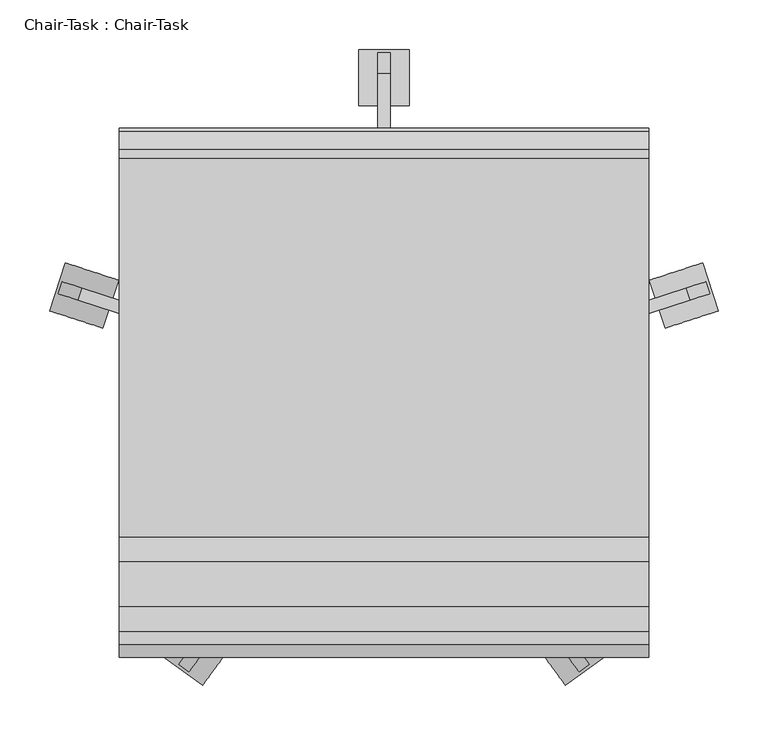
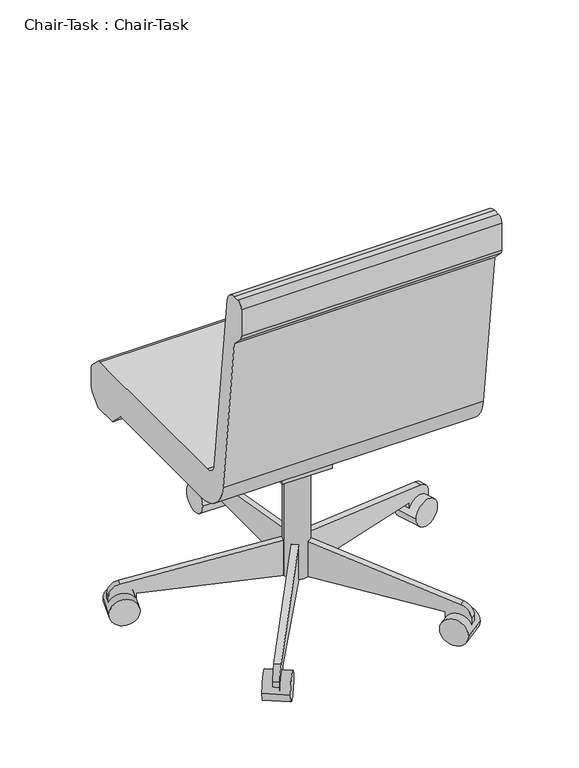
"""IFC4 building model written with IfcOpenShell, lengths in millimetres: furniture geometry, Chair-Task : Chair-Task."""

from ifc_helpers import new_model, si_unit, point, frame, frame_2d, origin, place, context, project, spatial, polyline, circle_curve, trimmed, segment, composite_curve, outline, extrude, source, transform, mapped, element, save


def chair_task_chair_task_b7f3823b(model_context):
    return source(origin(), model_context, "Body", "SweptSolid", [
        extrude(outline(composite_curve([segment(trimmed(circle_curve(frame_2d((140.9908197, 18.9459016)), 25.4), [point((115.5908197, 18.9459016))], [point((166.3908197, 18.9459016))], False, "CARTESIAN"), True, "CONTINUOUS"), segment(trimmed(circle_curve(frame_2d((140.9908197, 18.9459016)), 25.4), [point((166.3908197, 18.9459016))], [point((115.5908197, 18.9459016))], False, "CARTESIAN"), True, "CONTINUOUS")], self_intersect=False)), frame((0.0, 0.0, 53.5835944), z_axis=(0.0, 0.0, 1.0), x_axis=(1.0, 0.0, 0.0)), (0.0, 0.0, 1.0), 330.5914056),
        extrude(outline(composite_curve([segment(trimmed(circle_curve(frame_2d((0.0, -28.2002727)), 28.2002727), [point((0.0, -56.4005455))], [point((0.0, 0.0))], False, "CARTESIAN"), True, "CONTINUOUS"), segment(trimmed(circle_curve(frame_2d((0.0, -28.2002727)), 28.2002727), [point((0.0, 0.0))], [point((0.0, -56.4005455))], False, "CARTESIAN"), True, "CONTINUOUS")], self_intersect=False)), frame((477.6203484, 101.6163254, 28.1835944), z_axis=(-0.3090169943749423, 0.9510565162951553, 0.0), x_axis=(0.0, 0.0, 1.0)), (0.0, 0.0, 1.0), 50.8),
        extrude(outline(composite_curve([segment(polyline([(-25.4, 0.0), (0.0, 0.0), (0.0, -50.8), (-24.303053, -50.8)]), True, "CONTINUOUS"), segment(trimmed(circle_curve(frame_2d((-24.303053, -25.4)), 25.4), [point((-24.303053, -50.8))], [point((-49.3171699, -29.8106637))], False, "CARTESIAN"), True, "CONTINUOUS"), segment(polyline([(-49.3171699, -29.8106637), (-101.6, 266.7), (-101.6, 292.1), (-25.4, 292.1), (-25.4, 0.0)]), True, "CONTINUOUS")], self_intersect=False)), frame((420.756686, 103.1705568, 28.1835944), z_axis=(-0.3090169943749423, 0.9510565162951553, 0.0), x_axis=(0.0, 0.0, -1.0)), (0.0, 0.0, 1.0), 12.7),
        extrude(outline(composite_curve([segment(trimmed(circle_curve(frame_2d((0.0, -28.2002727)), 28.2002727), [point((0.0, -56.4005455))], [point((0.0, 0.0))], False, "CARTESIAN"), True, "CONTINUOUS"), segment(trimmed(circle_curve(frame_2d((0.0, -28.2002727)), 28.2002727), [point((0.0, 0.0))], [point((0.0, -56.4005455))], False, "CARTESIAN"), True, "CONTINUOUS")], self_intersect=False)), frame((323.63931, -275.6612394, 28.1835944), z_axis=(0.8090169943749499, 0.5877852522924699, 0.0), x_axis=(0.0, 0.0, 1.0)), (0.0, 0.0, 1.0), 50.8),
        extrude(outline(composite_curve([segment(polyline([(-25.4, 0.0), (0.0, 0.0), (0.0, -50.8), (-24.303053, -50.8)]), True, "CONTINUOUS"), segment(trimmed(circle_curve(frame_2d((-24.303053, -25.3999999)), 25.4), [point((-24.303053, -50.8))], [point((-49.3171699, -29.8106636))], False, "CARTESIAN"), True, "CONTINUOUS"), segment(polyline([(-49.3171699, -29.8106636), (-101.6, 266.7), (-101.6, 292.1), (-25.4, 292.1), (-25.4, 0.0)]), True, "CONTINUOUS")], self_intersect=False)), frame((307.545634, -221.1003988, 28.1835944), z_axis=(0.8090169943749499, 0.5877852522924699, 0.0), x_axis=(0.0, 0.0, -1.0)), (0.0, 0.0, 1.0), 12.7),
        extrude(outline(composite_curve([segment(trimmed(circle_curve(frame_2d((0.0, -28.2002727)), 28.2002727), [point((0.0, -56.4005455))], [point((0.0, 0.0))], False, "CARTESIAN"), True, "CONTINUOUS"), segment(trimmed(circle_curve(frame_2d((0.0, -28.2002727)), 28.2002727), [point((0.0, 0.0))], [point((0.0, -56.4005455))], False, "CARTESIAN"), True, "CONTINUOUS")], self_intersect=False)), frame((-41.6576707, -275.6612394, 28.1835944), z_axis=(-0.8090169943749458, 0.5877852522924754, 0.0), x_axis=(0.0, 0.0, -1.0)), (0.0, 0.0, 1.0), 50.8),
        extrude(outline(composite_curve([segment(polyline([(25.4, 0.0), (25.4, 292.1), (101.6, 292.1), (101.6, 266.7), (49.3171699, -29.8106637)]), True, "CONTINUOUS"), segment(trimmed(circle_curve(frame_2d((24.303053, -25.3999999)), 25.4), [point((49.3171699, -29.8106637))], [point((24.303053, -50.8))], False, "CARTESIAN"), True, "CONTINUOUS"), segment(polyline([(24.303053, -50.8), (0.0, -50.8), (0.0, 0.0), (25.4, 0.0)]), True, "CONTINUOUS")], self_intersect=False)), frame((-25.5639946, -221.1003988, 28.1835944), z_axis=(-0.8090169943749459, 0.5877852522924754, 0.0), x_axis=(0.0, 0.0, 1.0)), (0.0, 0.0, 1.0), 12.7),
        extrude(outline(composite_curve([segment(trimmed(circle_curve(frame_2d((0.0, -28.2002727)), 28.2002727), [point((0.0, -56.4005454))], [point((0.0, 0.0))], False, "CARTESIAN"), True, "CONTINUOUS"), segment(trimmed(circle_curve(frame_2d((0.0, -28.2002727)), 28.2002727), [point((0.0, 0.0))], [point((0.0, -56.4005454))], False, "CARTESIAN"), True, "CONTINUOUS")], self_intersect=False)), frame((-195.638709, 101.6163254, 28.1835944), z_axis=(0.3090169943749487, 0.9510565162951532, 0.0), x_axis=(0.0, 0.0, -1.0)), (0.0, 0.0, 1.0), 50.8),
        extrude(outline(composite_curve([segment(polyline([(25.4, 0.0), (25.4, 292.1000001), (101.6, 292.1000001), (101.6, 266.7), (49.3171699, -29.8106636)]), True, "CONTINUOUS"), segment(trimmed(circle_curve(frame_2d((24.303053, -25.4)), 25.4), [point((49.3171699, -29.8106636))], [point((24.303053, -50.8))], False, "CARTESIAN"), True, "CONTINUOUS"), segment(polyline([(24.303053, -50.8), (0.0, -50.8), (0.0, 0.0), (25.4, 0.0)]), True, "CONTINUOUS")], self_intersect=False)), frame((-138.7750467, 103.1705568, 28.1835944), z_axis=(0.3090169943749487, 0.9510565162951532, 0.0), x_axis=(0.0, 0.0, 1.0)), (0.0, 0.0, 1.0), 12.7),
        extrude(outline(composite_curve([segment(trimmed(circle_curve(frame_2d((336.4459016, 28.1835944)), 28.2002727), [point((308.2456289, 28.1835944))], [point((364.6461744, 28.1835944))], False, "CARTESIAN"), True, "CONTINUOUS"), segment(trimmed(circle_curve(frame_2d((336.4459016, 28.1835944)), 28.2002727), [point((364.6461744, 28.1835944))], [point((308.2456289, 28.1835944))], False, "CARTESIAN"), True, "CONTINUOUS")], self_intersect=False)), frame((115.5908197, 0.0, 0.0), z_axis=(1.0, 0.0, 0.0), x_axis=(0.0, 1.0, 0.0)), (0.0, 0.0, 1.0), 50.8),
        extrude(outline(composite_curve([segment(polyline([(311.0459016, 53.5835944), (18.9459016, 53.5835944), (18.9459016, 129.7835944), (44.3459016, 129.7835944), (340.8565654, 77.5007643)]), True, "CONTINUOUS"), segment(trimmed(circle_curve(frame_2d((336.4459016, 52.4866474)), 25.4), [point((340.8565654, 77.5007643))], [point((361.8459016, 52.4866474))], False, "CARTESIAN"), True, "CONTINUOUS"), segment(polyline([(361.8459016, 52.4866474), (361.8459016, 28.1835944), (311.0459016, 28.1835944), (311.0459016, 53.5835944)]), True, "CONTINUOUS")], self_intersect=False)), frame((134.6408197, 0.0, 0.0), z_axis=(1.0, 0.0, 0.0), x_axis=(0.0, 1.0, 0.0)), (0.0, 0.0, 1.0), 12.7),
        extrude(outline(polyline([(69.7459016, 383.7835944), (69.7459016, 371.0835944), (18.9459016, 283.0954134), (-19.1540984, 283.0954134), (-19.1540984, 383.7835944), (69.7459016, 383.7835944)])), frame((90.1908197, 0.0, 0.0), z_axis=(1.0, 0.0, 0.0), x_axis=(0.0, 1.0, 0.0)), (0.0, 0.0, 1.0), 101.6),
        extrude(outline(composite_curve([segment(polyline([(-126.2050455, 457.2), (255.0102301, 457.2)]), True, "CONTINUOUS"), segment(trimmed(circle_curve(frame_2d((255.0102301, 444.5)), 12.7), [point((255.0102301, 457.2))], [point((263.9604301, 453.510212))], False, "CARTESIAN"), True, "CONTINUOUS"), segment(polyline([(263.9604301, 453.510212), (281.8961016, 435.6939999)]), True, "CONTINUOUS"), segment(trimmed(circle_curve(frame_2d((272.9459016, 426.6837879)), 12.7), [point((281.8961016, 435.6939999))], [point((285.6459016, 426.6837879))], False, "CARTESIAN"), True, "CONTINUOUS"), segment(polyline([(285.6459016, 426.6837879), (285.6459016, 391.6405184)]), True, "CONTINUOUS"), segment(trimmed(circle_curve(frame_2d((260.2459016, 391.6405184)), 25.4), [point((285.6459016, 391.6405184))], [point((278.2663256, 373.7401184))], False, "CARTESIAN"), True, "CONTINUOUS"), segment(polyline([(278.2663256, 373.7401184), (260.2470284, 355.6), (209.4470284, 355.6), (181.0744602, 383.7835944), (-107.1089978, 383.7835944)]), True, "CONTINUOUS"), segment(trimmed(circle_curve(frame_2d((-107.1089978, 459.9835944)), 76.2), [point((-107.1089978, 383.7835944))], [point((-182.7870738, 451.0802913))], False, "CARTESIAN"), True, "CONTINUOUS"), segment(polyline([(-182.7870738, 451.0802913), (-222.3540984, 787.4), (-244.0343545, 809.0802561)]), True, "CONTINUOUS"), segment(trimmed(circle_curve(frame_2d((-235.0540984, 818.0605122)), 12.7), [point((-244.0343545, 809.0802561))], [point((-247.7540984, 818.0605122))], False, "CARTESIAN"), True, "CONTINUOUS"), segment(polyline([(-247.7540984, 818.0605122), (-247.7540984, 876.3)]), True, "CONTINUOUS"), segment(trimmed(circle_curve(frame_2d((-235.0540984, 876.3)), 12.7), [point((-247.7540984, 876.3))], [point((-235.0540984, 889.0))], False, "CARTESIAN"), True, "CONTINUOUS"), segment(polyline([(-235.0540984, 889.0), (-222.1789239, 889.0)]), True, "CONTINUOUS"), segment(trimmed(circle_curve(frame_2d((-222.1789239, 863.6)), 25.4), [point((-222.1789239, 889.0))], [point((-196.9528985, 866.5677677))], False, "CARTESIAN"), True, "CONTINUOUS"), segment(polyline([(-196.9528985, 866.5677677), (-151.4310708, 479.6322323)]), True, "CONTINUOUS"), segment(trimmed(circle_curve(frame_2d((-126.2050455, 482.6)), 25.4), [point((-151.4310708, 479.6322323))], [point((-126.2050455, 457.2))], True, "CARTESIAN"), True, "CONTINUOUS")], self_intersect=False)), frame((-125.7091803, 0.0, 0.0), z_axis=(1.0, 0.0, 0.0), x_axis=(0.0, 1.0, 0.0)), (0.0, 0.0, 1.0), 533.4),
    ])


if __name__ == "__main__":
    model = new_model("IFC4")
    model_context = context("Model", 3, world=origin())
    ifc_project = project(units=[si_unit("LENGTHUNIT", "METRE", prefix="MILLI")], contexts=[model_context])
    site = spatial("IfcSite", under=ifc_project)
    building = spatial("IfcBuilding", under=site)
    placement = place(None, origin())
    chair_task_chair_task_shape = chair_task_chair_task_b7f3823b(model_context)
    element("IfcFurniture", 1, ObjectType="Chair-Task : Chair-Task", at=placement, inside=building, context=model_context, shape_type="MappedRepresentation", body=[
        mapped(chair_task_chair_task_shape, transform((0.0, 0.0, 0.0), x_axis=(1.0, 0.0, 0.0), y_axis=(0.0, 1.0, 0.0), z_axis=(0.0, 0.0, 1.0))),
    ])
    save(model, "model.ifc")

# Revit data of these elements
# Type "Chair-Task : Chair-Task"
#   Assembly Code = "E2020200"
#   Base Material = Plastic - Black
#   Caster Material = Plastic - Black
#   Seat/Back Material = Textile - Slate Blue
#   Default Elevation = 0
# Element 1 (IfcFurniture, "Chair-Task : Chair-Task")
#   Materials on its faces: "Plastic - Black", "Textile - Slate Blue"
# Materials
#   "Plastic - Black": colour RGB 0 0 0, transparency 0.7
#   "Textile - Slate Blue": colour RGB 98 102 118, transparency 0
